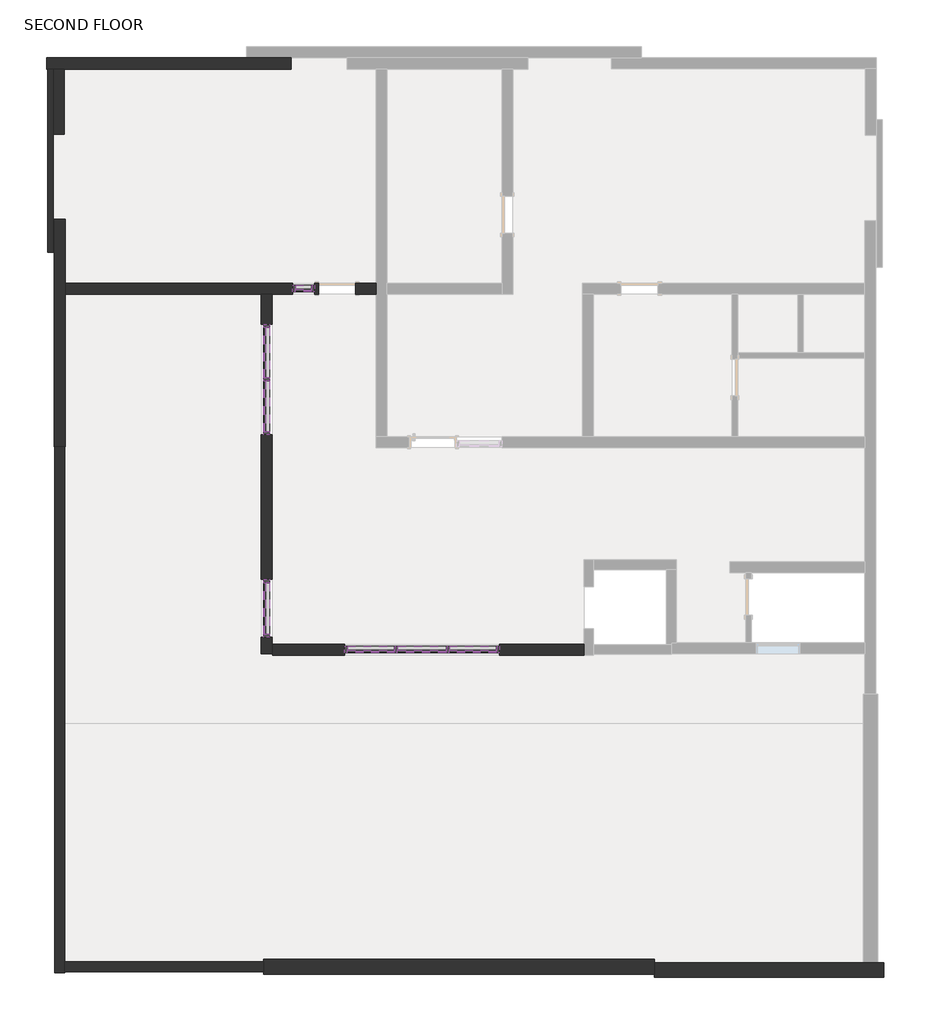
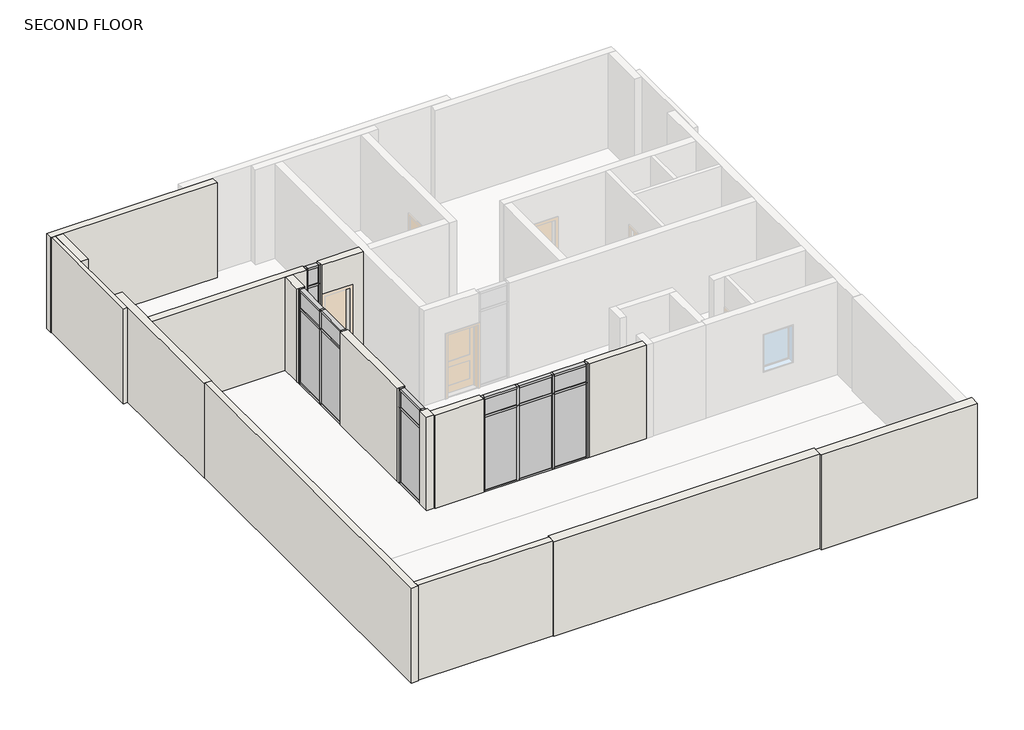
# One storey, part 1 of 2: 43 members, 14 plates, 11 walls.
"""IFC4 building model written with IfcOpenShell, lengths in millimetres."""

from ifc_helpers import new_model, si_unit, frame, origin, place, context, project, spatial, polyline, outline, extrude, faceted_brep, transform, mapped, element, save
from components import member_f0fea5a5, member_ee409385, member_c4de40ee, member_a715cb85, member_f03bb510, member_b0389538, member_0998ace5, member_b9dc02b9, member_6e77e263, member_47bfaf8a, member_78934672, member_697f972d, member_ff9f2d30, member_0c1408be, system_panel_glazed_daed1646, system_panel_glazed_43d75c16, system_panel_glazed_ee97838a, system_panel_glazed_b5d2153e, system_panel_glazed_ff9ba4bf, system_panel_glazed_ef7cd4ce, system_panel_glazed_cc935e45, system_panel_glazed_d41754d3, system_panel_glazed_720fdf88, system_panel_glazed_bfb04d77

model = new_model("IFC4")

# Units and contexts
model_context = context("Model", 3, world=origin())
ifc_project = project(units=[si_unit("LENGTHUNIT", "METRE", prefix="MILLI")], contexts=[model_context])

# Site, building, storey
site = spatial("IfcSite", under=ifc_project)
building = spatial("IfcBuilding", under=site)
storey = spatial("IfcBuildingStorey", under=building, Name="SECOND FLOOR", Elevation=6096.0)

# Members
placement = place(None, origin())
member_shape = member_f0fea5a5(model_context)
element("IfcMember", 1, ObjectType="Rectangular Mullion : 2.5\" x 5\" rectangular", at=placement, inside=storey, context=model_context, shape_type="MappedRepresentation", body=[
    mapped(member_shape, transform((2565.5464181, 4336.5216143, 6096.0), x_axis=(-1.0, 0.0, 0.0), y_axis=(0.0, 1.0, 0.0), z_axis=(0.0, 0.0, -1.0))),
])
element("IfcMember", 2, ObjectType="Rectangular Mullion : 2.5\" x 5\" rectangular", at=placement, inside=storey, context=model_context, shape_type="MappedRepresentation", body=[
    mapped(member_shape, transform((1498.7464183, 4336.5216143, 6096.0), x_axis=(-1.0, 0.0, 0.0), y_axis=(0.0, 1.0, 0.0), z_axis=(0.0, 0.0, -1.0))),
])
element("IfcMember", 3, ObjectType="Rectangular Mullion : 2.5\" x 5\" rectangular", at=placement, inside=storey, context=model_context, shape_type="MappedRepresentation", body=[
    mapped(member_shape, transform((-1181.6535114, 9915.8356247, 6096.0), x_axis=(0.0, 1.0, 0.0), y_axis=(1.0, 0.0, 0.0), z_axis=(0.0, 0.0, -1.0))),
])
member_2_shape = member_ee409385(model_context)
element("IfcMember", 4, ObjectType="Rectangular Mullion : 2.5\" x 5\" rectangular", at=placement, inside=storey, context=model_context, shape_type="MappedRepresentation", body=[
    mapped(member_2_shape, transform((431.9464182, 4336.5216143, 6096.0), x_axis=(-1.0, 0.0, 0.0), y_axis=(0.0, 1.0, 0.0), z_axis=(0.0, 0.0, -1.0))),
])
element("IfcMember", 5, ObjectType="Rectangular Mullion : 2.5\" x 5\" rectangular", at=placement, inside=storey, context=model_context, shape_type="MappedRepresentation", body=[
    mapped(member_2_shape, transform((-1181.6535114, 5784.3216143, 6096.0), x_axis=(0.0, 1.0, 0.0), y_axis=(1.0, 0.0, 0.0), z_axis=(0.0, 0.0, -1.0))),
])
element("IfcMember", 6, ObjectType="Rectangular Mullion : 2.5\" x 5\" rectangular", at=placement, inside=storey, context=model_context, shape_type="MappedRepresentation", body=[
    mapped(member_2_shape, transform((-1181.6535114, 11058.8356247, 6096.0), x_axis=(0.0, 1.0, 0.0), y_axis=(1.0, 0.0, 0.0), z_axis=(0.0, 0.0, -1.0))),
])
element("IfcMember", 7, ObjectType="Rectangular Mullion : 2.5\" x 5\" rectangular", at=placement, inside=storey, context=model_context, shape_type="MappedRepresentation", body=[
    mapped(member_2_shape, transform((-648.2535114, 11793.69348, 6096.0), x_axis=(-1.0, 0.0, 0.0), y_axis=(0.0, 1.0, 0.0), z_axis=(0.0, 0.0, -1.0))),
])
element("IfcMember", 8, ObjectType="Rectangular Mullion : 2.5\" x 5\" rectangular", at=placement, inside=storey, context=model_context, shape_type="MappedRepresentation", body=[
    mapped(member_2_shape, transform((3632.3464182, 4336.5216143, 8534.4), x_axis=(1.0, 0.0, 0.0), y_axis=(0.0, 1.0, 0.0), z_axis=(0.0, 0.0, 1.0))),
])
element("IfcMember", 9, ObjectType="Rectangular Mullion : 2.5\" x 5\" rectangular", at=placement, inside=storey, context=model_context, shape_type="MappedRepresentation", body=[
    mapped(member_2_shape, transform((-1181.6535114, 4590.5216143, 8534.4), x_axis=(0.0, -1.0, 0.0), y_axis=(1.0, 0.0, 0.0), z_axis=(0.0, 0.0, 1.0))),
])
element("IfcMember", 10, ObjectType="Rectangular Mullion : 2.5\" x 5\" rectangular", at=placement, inside=storey, context=model_context, shape_type="MappedRepresentation", body=[
    mapped(member_2_shape, transform((-1181.6535114, 8772.8356247, 8534.4), x_axis=(0.0, -1.0, 0.0), y_axis=(1.0, 0.0, 0.0), z_axis=(0.0, 0.0, 1.0))),
])
element("IfcMember", 11, ObjectType="Rectangular Mullion : 2.5\" x 5\" rectangular", at=placement, inside=storey, context=model_context, shape_type="MappedRepresentation", body=[
    mapped(member_2_shape, transform((-191.0535114, 11793.69348, 8534.4), x_axis=(1.0, 0.0, 0.0), y_axis=(0.0, 1.0, 0.0), z_axis=(0.0, 0.0, 1.0))),
])
member_3_shape = member_c4de40ee(model_context)
element("IfcMember", 12, ObjectType="Rectangular Mullion : 2.5\" x 5\" rectangular", at=placement, inside=storey, context=model_context, shape_type="MappedRepresentation", body=[
    mapped(member_3_shape, transform((-1181.6535114, 5720.8216143, 9144.0), x_axis=(0.0, 0.0, 1.0), y_axis=(1.0, 0.0, 0.0), z_axis=(0.0, 1.0, 0.0))),
])
element("IfcMember", 13, ObjectType="Rectangular Mullion : 2.5\" x 5\" rectangular", at=placement, inside=storey, context=model_context, shape_type="MappedRepresentation", body=[
    mapped(member_3_shape, transform((-1181.6535114, 4654.0216143, 6096.0), x_axis=(0.0, 0.0, -1.0), y_axis=(1.0, 0.0, 0.0), z_axis=(0.0, -1.0, 0.0))),
])
member_4_shape = member_a715cb85(model_context)
element("IfcMember", 14, ObjectType="Rectangular Mullion : 2.5\" x 5\" rectangular", at=placement, inside=storey, context=model_context, shape_type="MappedRepresentation", body=[
    mapped(member_4_shape, transform((-1181.6535114, 5720.8216143, 8534.4), x_axis=(0.0, 0.0, 1.0), y_axis=(1.0, 0.0, 0.0), z_axis=(0.0, 1.0, 0.0))),
])
member_5_shape = member_f03bb510(model_context)
element("IfcMember", 15, ObjectType="Rectangular Mullion : 2.5\" x 5\" rectangular", at=placement, inside=storey, context=model_context, shape_type="MappedRepresentation", body=[
    mapped(member_5_shape, transform((495.4464182, 4336.5216143, 9144.0), x_axis=(0.0, 0.0, 1.0), y_axis=(0.0, 1.0, 0.0), z_axis=(-1.0, 0.0, 0.0))),
])
element("IfcMember", 16, ObjectType="Rectangular Mullion : 2.5\" x 5\" rectangular", at=placement, inside=storey, context=model_context, shape_type="MappedRepresentation", body=[
    mapped(member_5_shape, transform((2597.2964181, 4336.5216143, 9144.0), x_axis=(0.0, 0.0, 1.0), y_axis=(0.0, 1.0, 0.0), z_axis=(-1.0, 0.0, 0.0))),
])
member_6_shape = member_b0389538(model_context)
element("IfcMember", 17, ObjectType="Rectangular Mullion : 2.5\" x 5\" rectangular", at=placement, inside=storey, context=model_context, shape_type="MappedRepresentation", body=[
    mapped(member_6_shape, transform((1530.4964183, 4336.5216143, 9144.0), x_axis=(0.0, 0.0, 1.0), y_axis=(0.0, 1.0, 0.0), z_axis=(-1.0, 0.0, 0.0))),
])
element("IfcMember", 18, ObjectType="Rectangular Mullion : 2.5\" x 5\" rectangular", at=placement, inside=storey, context=model_context, shape_type="MappedRepresentation", body=[
    mapped(member_5_shape, transform((3568.8464182, 4336.5216143, 6096.0), x_axis=(0.0, 0.0, -1.0), y_axis=(0.0, 1.0, 0.0), z_axis=(1.0, 0.0, 0.0))),
])
element("IfcMember", 19, ObjectType="Rectangular Mullion : 2.5\" x 5\" rectangular", at=placement, inside=storey, context=model_context, shape_type="MappedRepresentation", body=[
    mapped(member_5_shape, transform((1466.9964183, 4336.5216143, 6096.0), x_axis=(0.0, 0.0, -1.0), y_axis=(0.0, 1.0, 0.0), z_axis=(1.0, 0.0, 0.0))),
])
element("IfcMember", 20, ObjectType="Rectangular Mullion : 2.5\" x 5\" rectangular", at=placement, inside=storey, context=model_context, shape_type="MappedRepresentation", body=[
    mapped(member_6_shape, transform((2533.7964181, 4336.5216143, 6096.0), x_axis=(0.0, 0.0, -1.0), y_axis=(0.0, 1.0, 0.0), z_axis=(1.0, 0.0, 0.0))),
])
member_7_shape = member_0998ace5(model_context)
element("IfcMember", 21, ObjectType="Rectangular Mullion : 2.5\" x 5\" rectangular", at=placement, inside=storey, context=model_context, shape_type="MappedRepresentation", body=[
    mapped(member_7_shape, transform((2597.2964181, 4336.5216143, 8534.4), x_axis=(0.0, 0.0, 1.0), y_axis=(0.0, 1.0, 0.0), z_axis=(-1.0, 0.0, 0.0))),
])
element("IfcMember", 22, ObjectType="Rectangular Mullion : 2.5\" x 5\" rectangular", at=placement, inside=storey, context=model_context, shape_type="MappedRepresentation", body=[
    mapped(member_7_shape, transform((495.4464182, 4336.5216143, 8534.4), x_axis=(0.0, 0.0, 1.0), y_axis=(0.0, 1.0, 0.0), z_axis=(-1.0, 0.0, 0.0))),
])
member_8_shape = member_b9dc02b9(model_context)
element("IfcMember", 23, ObjectType="Rectangular Mullion : 2.5\" x 5\" rectangular", at=placement, inside=storey, context=model_context, shape_type="MappedRepresentation", body=[
    mapped(member_8_shape, transform((1530.4964183, 4336.5216143, 8534.4), x_axis=(0.0, 0.0, 1.0), y_axis=(0.0, 1.0, 0.0), z_axis=(-1.0, 0.0, 0.0))),
])
member_9_shape = member_6e77e263(model_context)
element("IfcMember", 24, ObjectType="Rectangular Mullion : 2.5\" x 5\" rectangular", at=placement, inside=storey, context=model_context, shape_type="MappedRepresentation", body=[
    mapped(member_9_shape, transform((2565.5464181, 4336.5216143, 8534.4), x_axis=(-1.0, 0.0, 0.0), y_axis=(0.0, 1.0, 0.0), z_axis=(0.0, 0.0, -1.0))),
])
element("IfcMember", 25, ObjectType="Rectangular Mullion : 2.5\" x 5\" rectangular", at=placement, inside=storey, context=model_context, shape_type="MappedRepresentation", body=[
    mapped(member_9_shape, transform((1498.7464183, 4336.5216143, 8534.4), x_axis=(-1.0, 0.0, 0.0), y_axis=(0.0, 1.0, 0.0), z_axis=(0.0, 0.0, -1.0))),
])
element("IfcMember", 26, ObjectType="Rectangular Mullion : 2.5\" x 5\" rectangular", at=placement, inside=storey, context=model_context, shape_type="MappedRepresentation", body=[
    mapped(member_9_shape, transform((-1181.6535114, 9915.8356247, 8534.4), x_axis=(0.0, 1.0, 0.0), y_axis=(1.0, 0.0, 0.0), z_axis=(0.0, 0.0, -1.0))),
])
member_10_shape = member_47bfaf8a(model_context)
element("IfcMember", 27, ObjectType="Rectangular Mullion : 2.5\" x 5\" rectangular", at=placement, inside=storey, context=model_context, shape_type="MappedRepresentation", body=[
    mapped(member_10_shape, transform((431.9464182, 4336.5216143, 8534.4), x_axis=(-1.0, 0.0, 0.0), y_axis=(0.0, 1.0, 0.0), z_axis=(0.0, 0.0, -1.0))),
])
element("IfcMember", 28, ObjectType="Rectangular Mullion : 2.5\" x 5\" rectangular", at=placement, inside=storey, context=model_context, shape_type="MappedRepresentation", body=[
    mapped(member_10_shape, transform((-1181.6535114, 5784.3216143, 8534.4), x_axis=(0.0, 1.0, 0.0), y_axis=(1.0, 0.0, 0.0), z_axis=(0.0, 0.0, -1.0))),
])
element("IfcMember", 29, ObjectType="Rectangular Mullion : 2.5\" x 5\" rectangular", at=placement, inside=storey, context=model_context, shape_type="MappedRepresentation", body=[
    mapped(member_10_shape, transform((-1181.6535114, 11058.8356247, 8534.4), x_axis=(0.0, 1.0, 0.0), y_axis=(1.0, 0.0, 0.0), z_axis=(0.0, 0.0, -1.0))),
])
element("IfcMember", 30, ObjectType="Rectangular Mullion : 2.5\" x 5\" rectangular", at=placement, inside=storey, context=model_context, shape_type="MappedRepresentation", body=[
    mapped(member_10_shape, transform((-648.2535114, 11793.69348, 8534.4), x_axis=(-1.0, 0.0, 0.0), y_axis=(0.0, 1.0, 0.0), z_axis=(0.0, 0.0, -1.0))),
])
element("IfcMember", 31, ObjectType="Rectangular Mullion : 2.5\" x 5\" rectangular", at=placement, inside=storey, context=model_context, shape_type="MappedRepresentation", body=[
    mapped(member_10_shape, transform((3632.3464182, 4336.5216143, 9144.0), x_axis=(1.0, 0.0, 0.0), y_axis=(0.0, 1.0, 0.0), z_axis=(0.0, 0.0, 1.0))),
])
element("IfcMember", 32, ObjectType="Rectangular Mullion : 2.5\" x 5\" rectangular", at=placement, inside=storey, context=model_context, shape_type="MappedRepresentation", body=[
    mapped(member_10_shape, transform((-1181.6535114, 4590.5216143, 9144.0), x_axis=(0.0, -1.0, 0.0), y_axis=(1.0, 0.0, 0.0), z_axis=(0.0, 0.0, 1.0))),
])
element("IfcMember", 33, ObjectType="Rectangular Mullion : 2.5\" x 5\" rectangular", at=placement, inside=storey, context=model_context, shape_type="MappedRepresentation", body=[
    mapped(member_10_shape, transform((-1181.6535114, 8772.8356247, 9144.0), x_axis=(0.0, -1.0, 0.0), y_axis=(1.0, 0.0, 0.0), z_axis=(0.0, 0.0, 1.0))),
])
element("IfcMember", 34, ObjectType="Rectangular Mullion : 2.5\" x 5\" rectangular", at=placement, inside=storey, context=model_context, shape_type="MappedRepresentation", body=[
    mapped(member_10_shape, transform((-191.0535114, 11793.69348, 9144.0), x_axis=(1.0, 0.0, 0.0), y_axis=(0.0, 1.0, 0.0), z_axis=(0.0, 0.0, 1.0))),
])
member_11_shape = member_78934672(model_context)
element("IfcMember", 35, ObjectType="Rectangular Mullion : 2.5\" x 5\" rectangular", at=placement, inside=storey, context=model_context, shape_type="MappedRepresentation", body=[
    mapped(member_11_shape, transform((-1181.6535114, 10995.3356247, 9144.0), x_axis=(0.0, 0.0, 1.0), y_axis=(1.0, 0.0, 0.0), z_axis=(0.0, 1.0, 0.0))),
])
element("IfcMember", 36, ObjectType="Rectangular Mullion : 2.5\" x 5\" rectangular", at=placement, inside=storey, context=model_context, shape_type="MappedRepresentation", body=[
    mapped(member_11_shape, transform((-1181.6535114, 9884.0856247, 9144.0), x_axis=(0.0, 0.0, 1.0), y_axis=(1.0, 0.0, 0.0), z_axis=(0.0, 1.0, 0.0))),
])
element("IfcMember", 37, ObjectType="Rectangular Mullion : 2.5\" x 5\" rectangular", at=placement, inside=storey, context=model_context, shape_type="MappedRepresentation", body=[
    mapped(member_11_shape, transform((-1181.6535114, 8836.3356247, 6096.0), x_axis=(0.0, 0.0, -1.0), y_axis=(1.0, 0.0, 0.0), z_axis=(0.0, -1.0, 0.0))),
])
element("IfcMember", 38, ObjectType="Rectangular Mullion : 2.5\" x 5\" rectangular", at=placement, inside=storey, context=model_context, shape_type="MappedRepresentation", body=[
    mapped(member_11_shape, transform((-1181.6535114, 9947.5856247, 6096.0), x_axis=(0.0, 0.0, -1.0), y_axis=(1.0, 0.0, 0.0), z_axis=(0.0, -1.0, 0.0))),
])
member_12_shape = member_697f972d(model_context)
element("IfcMember", 39, ObjectType="Rectangular Mullion : 2.5\" x 5\" rectangular", at=placement, inside=storey, context=model_context, shape_type="MappedRepresentation", body=[
    mapped(member_12_shape, transform((-1181.6535114, 9884.0856247, 8534.4), x_axis=(0.0, 0.0, 1.0), y_axis=(1.0, 0.0, 0.0), z_axis=(0.0, 1.0, 0.0))),
])
element("IfcMember", 40, ObjectType="Rectangular Mullion : 2.5\" x 5\" rectangular", at=placement, inside=storey, context=model_context, shape_type="MappedRepresentation", body=[
    mapped(member_12_shape, transform((-1181.6535114, 10995.3356247, 8534.4), x_axis=(0.0, 0.0, 1.0), y_axis=(1.0, 0.0, 0.0), z_axis=(0.0, 1.0, 0.0))),
])
member_13_shape = member_ff9f2d30(model_context)
element("IfcMember", 41, ObjectType="Rectangular Mullion : 2.5\" x 5\" rectangular", at=placement, inside=storey, context=model_context, shape_type="MappedRepresentation", body=[
    mapped(member_13_shape, transform((-584.7535114, 11793.69348, 9144.0), x_axis=(0.0, 0.0, 1.0), y_axis=(0.0, 1.0, 0.0), z_axis=(-1.0, 0.0, 0.0))),
])
element("IfcMember", 42, ObjectType="Rectangular Mullion : 2.5\" x 5\" rectangular", at=placement, inside=storey, context=model_context, shape_type="MappedRepresentation", body=[
    mapped(member_13_shape, transform((-254.5535114, 11793.69348, 6096.0), x_axis=(0.0, 0.0, -1.0), y_axis=(0.0, 1.0, 0.0), z_axis=(1.0, 0.0, 0.0))),
])
member_14_shape = member_0c1408be(model_context)
element("IfcMember", 43, ObjectType="Rectangular Mullion : 2.5\" x 5\" rectangular", at=placement, inside=storey, context=model_context, shape_type="MappedRepresentation", body=[
    mapped(member_14_shape, transform((-584.7535114, 11793.69348, 8534.4), x_axis=(0.0, 0.0, 1.0), y_axis=(0.0, 1.0, 0.0), z_axis=(-1.0, 0.0, 0.0))),
])

# Plates
system_panel_glazed_shape = system_panel_glazed_daed1646(model_context)
element("IfcPlate", 44, ObjectType="System Panel : Glazed", at=placement, inside=storey, context=model_context, shape_type="MappedRepresentation", body=[
    mapped(system_panel_glazed_shape, transform((-1181.6535114, 5187.4216143, 6159.5), x_axis=(0.0, 1.0, 0.0), y_axis=(-1.0, 0.0, 0.0), z_axis=(0.0, 0.0, 1.0))),
])
system_panel_glazed_2_shape = system_panel_glazed_43d75c16(model_context)
element("IfcPlate", 45, ObjectType="System Panel : Glazed", at=placement, inside=storey, context=model_context, shape_type="MappedRepresentation", body=[
    mapped(system_panel_glazed_2_shape, transform((3083.0714181, 4336.5216143, 6159.5), x_axis=(-1.0, 0.0, 0.0), y_axis=(0.0, -1.0, 0.0), z_axis=(0.0, 0.0, 1.0))),
])
element("IfcPlate", 46, ObjectType="System Panel : Glazed", at=placement, inside=storey, context=model_context, shape_type="MappedRepresentation", body=[
    mapped(system_panel_glazed_2_shape, transform((981.2214182, 4336.5216143, 6159.5), x_axis=(-1.0, 0.0, 0.0), y_axis=(0.0, -1.0, 0.0), z_axis=(0.0, 0.0, 1.0))),
])
system_panel_glazed_3_shape = system_panel_glazed_ee97838a(model_context)
element("IfcPlate", 47, ObjectType="System Panel : Glazed", at=placement, inside=storey, context=model_context, shape_type="MappedRepresentation", body=[
    mapped(system_panel_glazed_3_shape, transform((2032.1464182, 4336.5216143, 6159.5), x_axis=(-1.0, 0.0, 0.0), y_axis=(0.0, -1.0, 0.0), z_axis=(0.0, 0.0, 1.0))),
])
system_panel_glazed_4_shape = system_panel_glazed_b5d2153e(model_context)
element("IfcPlate", 48, ObjectType="System Panel : Glazed", at=placement, inside=storey, context=model_context, shape_type="MappedRepresentation", body=[
    mapped(system_panel_glazed_4_shape, transform((3083.0714181, 4336.5216143, 8566.15), x_axis=(-1.0, 0.0, 0.0), y_axis=(0.0, -1.0, 0.0), z_axis=(0.0, 0.0, 1.0))),
])
element("IfcPlate", 49, ObjectType="System Panel : Glazed", at=placement, inside=storey, context=model_context, shape_type="MappedRepresentation", body=[
    mapped(system_panel_glazed_4_shape, transform((981.2214182, 4336.5216143, 8566.15), x_axis=(-1.0, 0.0, 0.0), y_axis=(0.0, -1.0, 0.0), z_axis=(0.0, 0.0, 1.0))),
])
system_panel_glazed_5_shape = system_panel_glazed_ff9ba4bf(model_context)
element("IfcPlate", 50, ObjectType="System Panel : Glazed", at=placement, inside=storey, context=model_context, shape_type="MappedRepresentation", body=[
    mapped(system_panel_glazed_5_shape, transform((2032.1464182, 4336.5216143, 8566.15), x_axis=(-1.0, 0.0, 0.0), y_axis=(0.0, -1.0, 0.0), z_axis=(0.0, 0.0, 1.0))),
])
system_panel_glazed_6_shape = system_panel_glazed_ef7cd4ce(model_context)
element("IfcPlate", 51, ObjectType="System Panel : Glazed", at=placement, inside=storey, context=model_context, shape_type="MappedRepresentation", body=[
    mapped(system_panel_glazed_6_shape, transform((-1181.6535114, 5187.4216143, 8566.15), x_axis=(0.0, 1.0, 0.0), y_axis=(-1.0, 0.0, 0.0), z_axis=(0.0, 0.0, 1.0))),
])
system_panel_glazed_7_shape = system_panel_glazed_cc935e45(model_context)
element("IfcPlate", 52, ObjectType="System Panel : Glazed", at=placement, inside=storey, context=model_context, shape_type="MappedRepresentation", body=[
    mapped(system_panel_glazed_7_shape, transform((-1181.6535114, 9360.2106247, 6159.5), x_axis=(0.0, 1.0, 0.0), y_axis=(-1.0, 0.0, 0.0), z_axis=(0.0, 0.0, 1.0))),
])
element("IfcPlate", 53, ObjectType="System Panel : Glazed", at=placement, inside=storey, context=model_context, shape_type="MappedRepresentation", body=[
    mapped(system_panel_glazed_7_shape, transform((-1181.6535114, 10471.4606247, 6159.5), x_axis=(0.0, 1.0, 0.0), y_axis=(-1.0, 0.0, 0.0), z_axis=(0.0, 0.0, 1.0))),
])
system_panel_glazed_8_shape = system_panel_glazed_d41754d3(model_context)
element("IfcPlate", 54, ObjectType="System Panel : Glazed", at=placement, inside=storey, context=model_context, shape_type="MappedRepresentation", body=[
    mapped(system_panel_glazed_8_shape, transform((-1181.6535114, 9360.2106247, 8566.15), x_axis=(0.0, 1.0, 0.0), y_axis=(-1.0, 0.0, 0.0), z_axis=(0.0, 0.0, 1.0))),
])
element("IfcPlate", 55, ObjectType="System Panel : Glazed", at=placement, inside=storey, context=model_context, shape_type="MappedRepresentation", body=[
    mapped(system_panel_glazed_8_shape, transform((-1181.6535114, 10471.4606247, 8566.15), x_axis=(0.0, 1.0, 0.0), y_axis=(-1.0, 0.0, 0.0), z_axis=(0.0, 0.0, 1.0))),
])
system_panel_glazed_9_shape = system_panel_glazed_720fdf88(model_context)
element("IfcPlate", 56, ObjectType="System Panel : Glazed", at=placement, inside=storey, context=model_context, shape_type="MappedRepresentation", body=[
    mapped(system_panel_glazed_9_shape, transform((-419.6535114, 11793.69348, 6159.5), x_axis=(-1.0, 0.0, 0.0), y_axis=(0.0, -1.0, 0.0), z_axis=(0.0, 0.0, 1.0))),
])
system_panel_glazed_10_shape = system_panel_glazed_bfb04d77(model_context)
element("IfcPlate", 57, ObjectType="System Panel : Glazed", at=placement, inside=storey, context=model_context, shape_type="MappedRepresentation", body=[
    mapped(system_panel_glazed_10_shape, transform((-419.6535114, 11793.69348, 8566.15), x_axis=(-1.0, 0.0, 0.0), y_axis=(0.0, -1.0, 0.0), z_axis=(0.0, 0.0, 1.0))),
])

# Walls
element("IfcWall", 58, ObjectType="INNER WALL 4.5\"", at=placement, inside=storey, context=model_context, shape_type="SweptSolid", body=[
    extrude(outline(polyline([(-5594.7327494, 16327.59348), (-5594.7327494, 12547.6213266), (-5709.0327494, 12547.6213266), (-5709.0327494, 16327.59348), (-5594.7327494, 16327.59348)])), frame((0.0, 0.0, 6096.0), z_axis=(0.0, 0.0, 1.0), x_axis=(1.0, 0.0, 0.0)), (0.0, 0.0, 1.0), 3048.0),
])
element("IfcWall", 59, ObjectType="OUTER WALL THICKNESS 8\"", at=placement, inside=storey, context=model_context, shape_type="Brep", body=[
    faceted_brep([(-5560.894009, 8528.9097639, 6096.0), (-5560.894009, -2342.2902361, 6096.0), (-5560.894009, -2342.2902361, 9144.0), (-5560.894009, 8528.9097639, 9144.0), (-5357.694009, 8528.9097639, 6096.0), (-5357.694009, 8528.9097639, 9144.0), (-5357.694009, -2113.6902361, 9144.0), (-5357.694009, -2316.8902361, 9144.0), (-5357.694009, -2342.2902361, 9144.0), (-5357.694009, -2342.2902361, 6096.0), (-5357.694009, -2316.8902361, 6096.0), (-5357.694009, -2113.6902361, 6096.0)], [[[0, 1, 2, 3]], [[4, 5, 6, 7, 8, 9, 10, 11]], [[1, 0, 4, 11, 10, 9]], [[2, 1, 9, 8]], [[3, 2, 8, 7, 6, 5]], [[0, 3, 5, 4]]]),
])
element("IfcWall", 60, ObjectType="OUTER WALL THICKNESS 8\"", at=placement, inside=storey, context=model_context, shape_type="SweptSolid", body=[
    extrude(outline(polyline([(-1242.894009, -2316.8902361), (-5357.694009, -2316.8902361), (-5357.694009, -2113.6902361), (-1242.894009, -2113.6902361), (-1242.894009, -2316.8902361)])), frame((0.0, 0.0, 6096.0), z_axis=(0.0, 0.0, 1.0), x_axis=(1.0, 0.0, 0.0)), (0.0, 0.0, 1.0), 3048.0),
])
element("IfcWall", 61, ObjectType="OUTER WALL THICKNESS 9\"", at=placement, inside=storey, context=model_context, shape_type="Brep", body=[
    faceted_brep([(-674.5187543, 16556.19348, 6096.0), (-5729.1187543, 16556.19348, 6096.0), (-5729.1187543, 16556.19348, 9144.0), (-674.5187543, 16556.19348, 9144.0), (-674.5187543, 16327.59348, 6096.0), (-674.5187543, 16327.59348, 9144.0), (-5364.044009, 16327.59348, 9144.0), (-5592.644009, 16327.59348, 9144.0), (-5594.7327494, 16327.59348, 9144.0), (-5709.0327494, 16327.59348, 9144.0), (-5729.1187543, 16327.59348, 9144.0), (-5729.1187543, 16327.59348, 6096.0), (-5709.0327494, 16327.59348, 6096.0), (-5594.7327494, 16327.59348, 6096.0), (-5592.644009, 16327.59348, 6096.0), (-5364.044009, 16327.59348, 6096.0)], [[[0, 1, 2, 3]], [[4, 5, 6, 7, 8, 9, 10, 11, 12, 13, 14, 15]], [[1, 0, 4, 15, 14, 13, 12, 11]], [[2, 1, 11, 10]], [[3, 2, 10, 9, 8, 7, 6, 5]], [[0, 3, 5, 4]]]),
])
element("IfcWall", 62, ObjectType="OUTER WALL THICKNESS 9\"", at=placement, inside=storey, context=model_context, shape_type="SweptSolid", body=[
    extrude(outline(polyline([(-5592.644009, 14981.39348), (-5592.644009, 16327.59348), (-5364.044009, 16327.59348), (-5364.044009, 14981.39348), (-5592.644009, 14981.39348)])), frame((0.0, 0.0, 6096.0), z_axis=(0.0, 0.0, 1.0), x_axis=(1.0, 0.0, 0.0)), (0.0, 0.0, 1.0), 3048.0),
])
element("IfcWall", 63, ObjectType="OUTER WALL THICKNESS 9\"", at=placement, inside=storey, context=model_context, shape_type="Brep", body=[
    faceted_brep([(-5573.594009, 13227.9097639, 6096.0), (-5573.594009, 8528.9097639, 6096.0), (-5573.594009, 8528.9097639, 9144.0), (-5573.594009, 13227.9097639, 9144.0), (-5344.994009, 13227.9097639, 6096.0), (-5344.994009, 13227.9097639, 9144.0), (-5344.994009, 11907.99348, 9144.0), (-5344.994009, 11679.39348, 9144.0), (-5344.994009, 8528.9097639, 9144.0), (-5344.994009, 8528.9097639, 6096.0), (-5344.994009, 11679.39348, 6096.0), (-5344.994009, 11907.99348, 6096.0), (-5357.694009, 8528.9097639, 6096.0), (-5560.894009, 8528.9097639, 6096.0), (-5357.694009, 8528.9097639, 9144.0), (-5560.894009, 8528.9097639, 9144.0)], [[[0, 1, 2, 3]], [[4, 5, 6, 7, 8, 9, 10, 11]], [[1, 0, 4, 11, 10, 9, 12, 13]], [[2, 1, 13, 12, 9, 8, 14, 15]], [[3, 2, 15, 14, 8, 7, 6, 5]], [[0, 3, 5, 4]]]),
])
element("IfcWall", 64, ObjectType="OUTER WALL THICKNESS 9\"", at=placement, inside=storey, context=model_context, shape_type="Brep", body=[
    faceted_brep([(1076.9068953, 11679.39348, 6096.0), (1076.9068953, 11679.39348, 9144.0), (-191.0535114, 11679.39348, 9144.0), (-191.0535114, 11679.39348, 6096.0), (-104.1931047, 11679.39348, 6096.0), (-104.1931047, 11679.39348, 8128.0), (657.8068953, 11679.39348, 8128.0), (657.8068953, 11679.39348, 6096.0), (1076.9068953, 11907.99348, 9144.0), (1076.9068953, 11907.99348, 6096.0), (657.8068953, 11907.99348, 6096.0), (657.8068953, 11907.99348, 8128.0), (-104.1931047, 11907.99348, 8128.0), (-104.1931047, 11907.99348, 6096.0), (-191.0535114, 11907.99348, 6096.0), (-191.0535114, 11907.99348, 9144.0)], [[[0, 1, 2, 3, 4, 5, 6, 7]], [[8, 9, 10, 11, 12, 13, 14, 15]], [[9, 0, 7, 10]], [[13, 4, 3, 14]], [[1, 8, 15, 2]], [[1, 0, 9, 8]], [[11, 10, 7, 6]], [[12, 11, 6, 5]], [[13, 12, 5, 4]], [[3, 2, 15, 14]]]),
    faceted_brep([(-5344.994009, 11679.39348, 9144.0), (-5344.994009, 11679.39348, 6096.0), (-1295.9535114, 11679.39348, 6096.0), (-1067.3535114, 11679.39348, 6096.0), (-648.2535114, 11679.39348, 6096.0), (-648.2535114, 11679.39348, 9144.0), (-1067.3535114, 11679.39348, 9144.0), (-1295.9535114, 11679.39348, 9144.0), (-5344.994009, 11907.99348, 6096.0), (-5344.994009, 11907.99348, 9144.0), (-648.2535114, 11907.99348, 9144.0), (-648.2535114, 11907.99348, 6096.0)], [[[0, 1, 2, 3, 4, 5, 6, 7]], [[8, 9, 10, 11]], [[1, 8, 11, 4, 3, 2]], [[9, 0, 7, 6, 5, 10]], [[1, 0, 9, 8]], [[5, 4, 11, 10]]]),
])
element("IfcWall", 65, ObjectType="OUTER WALL THICKNESS 9\"", at=placement, inside=storey, context=model_context, shape_type="SweptSolid", body=[
    extrude(outline(polyline([(-1067.3535114, 4249.89348), (-1295.9535114, 4249.89348), (-1295.9535114, 4590.5216143), (-1067.3535114, 4590.5216143), (-1067.3535114, 4249.89348)])), frame((0.0, 0.0, 6096.0), z_axis=(0.0, 0.0, 1.0), x_axis=(1.0, 0.0, 0.0)), (0.0, 0.0, 1.0), 3048.0),
    extrude(outline(polyline([(-1295.9535114, 11679.39348), (-1067.3535114, 11679.39348), (-1067.3535114, 11058.8356247), (-1295.9535114, 11058.8356247), (-1295.9535114, 11679.39348)])), frame((0.0, 0.0, 6096.0), z_axis=(0.0, 0.0, 1.0), x_axis=(1.0, 0.0, 0.0)), (0.0, 0.0, 1.0), 3048.0),
    extrude(outline(polyline([(-1067.3535114, 5784.3216143), (-1295.9535114, 5784.3216143), (-1295.9535114, 8772.8356247), (-1067.3535114, 8772.8356247), (-1067.3535114, 5784.3216143)])), frame((0.0, 0.0, 6096.0), z_axis=(0.0, 0.0, 1.0), x_axis=(1.0, 0.0, 0.0)), (0.0, 0.0, 1.0), 3048.0),
])
element("IfcWall", 66, ObjectType="OUTER WALL THICKNESS 9\"", at=placement, inside=storey, context=model_context, shape_type="SweptSolid", body=[
    extrude(outline(polyline([(-1059.3262442, 4222.2216143), (-1059.3262442, 4450.8216143), (431.9464182, 4450.8216143), (431.9464182, 4222.2216143), (-1059.3262442, 4222.2216143)])), frame((0.0, 0.0, 6096.0), z_axis=(0.0, 0.0, 1.0), x_axis=(1.0, 0.0, 0.0)), (0.0, 0.0, 1.0), 3048.0),
    extrude(outline(polyline([(5375.3606323, 4450.8216143), (5375.3606323, 4222.2216143), (3632.3464182, 4222.2216143), (3632.3464182, 4450.8216143), (5375.3606323, 4450.8216143)])), frame((0.0, 0.0, 6096.0), z_axis=(0.0, 0.0, 1.0), x_axis=(1.0, 0.0, 0.0)), (0.0, 0.0, 1.0), 3048.0),
])
element("IfcWall", 67, ObjectType="WALL THICKNESS 1'", at=placement, inside=storey, context=model_context, shape_type="Brep", body=[
    faceted_brep([(-1242.894009, -2367.6902361, 6096.0), (6834.305991, -2367.6902361, 6096.0), (6834.305991, -2367.6902361, 9144.0), (-1242.894009, -2367.6902361, 9144.0), (-1242.894009, -2062.8902361, 6096.0), (-1242.894009, -2062.8902361, 9144.0), (6834.305991, -2062.8902361, 9144.0), (6834.305991, -2062.8902361, 6096.0), (-1242.894009, -2316.8902361, 6096.0), (-1242.894009, -2113.6902361, 6096.0), (6834.305991, -2132.117542, 6096.0), (6834.305991, -2132.117542, 9144.0), (-1242.894009, -2113.6902361, 9144.0), (-1242.894009, -2316.8902361, 9144.0)], [[[0, 1, 2, 3]], [[4, 5, 6, 7]], [[1, 0, 8, 9, 4, 7, 10]], [[2, 1, 10, 7, 6, 11]], [[3, 2, 11, 6, 5, 12, 13]], [[0, 3, 13, 12, 5, 4, 9, 8]]]),
])
element("IfcWall", 68, ObjectType="WALL THICKNESS 1'", at=placement, inside=storey, context=model_context, shape_type="Brep", body=[
    faceted_brep([(6834.305991, -2436.917542, 6096.0), (11579.9862453, -2436.917542, 6096.0), (11579.9862453, -2436.917542, 9144.0), (6834.305991, -2436.917542, 9144.0), (6834.305991, -2132.117542, 6096.0), (6834.305991, -2132.117542, 9144.0), (11147.3141504, -2132.117542, 9144.0), (11452.1141504, -2132.117542, 9144.0), (11579.9862453, -2132.117542, 9144.0), (11579.9862453, -2132.117542, 6096.0), (11452.1141504, -2132.117542, 6096.0), (11147.3141504, -2132.117542, 6096.0), (6834.305991, -2367.6902361, 6096.0), (6834.305991, -2367.6902361, 9144.0)], [[[0, 1, 2, 3]], [[4, 5, 6, 7, 8, 9, 10, 11]], [[1, 0, 12, 4, 11, 10, 9]], [[2, 1, 9, 8]], [[3, 2, 8, 7, 6, 5, 13]], [[0, 3, 13, 5, 4, 12]]]),
])

save(model, "model.ifc")

# Revit data of these elements
# Type "Rectangular Mullion : 2.5\" x 5\" rectangular"
#   built-in parameter 1007304 = 0.416667 (stored number, unit not read)
#   built-in parameter 1007301 = 0.104167 (stored number, unit not read)
#   built-in parameter 1007300 = 0.104167 (stored number, unit not read)
# Type "System Panel : Glazed"
#   Construction Type Id = "GSP4R"
#   Analytic Construction = "1/8 in Pilkington single glazing"
#   Visual Light Transmittance = 0.9
#   Solar Heat Gain Coefficient = 0.86
#   Heat Transfer Coefficient (U) = 1.18115 BTU/(h·ft²·°F)
#   Define Thermal Properties by = 1
# Type "INNER WALL 4.5\""
#   Assembly Code = "B2010"
#   Layers, outside or top first: 0' - 4 1/2" "BEIGE COLOUR" (function 1)
# Type "OUTER WALL THICKNESS 8\""
#   Assembly Code = "B2010"
#   Layers, outside or top first: 0' - 8" "BEIGE COLOUR" (function 1)
# Type "OUTER WALL THICKNESS 9\""
#   Assembly Code = "B2010"
#   Layers, outside or top first: 0' - 9" "BEIGE COLOUR" (function 1)
# Type "WALL THICKNESS 1'"
#   Assembly Code = "B2010"
#   Layers, outside or top first: 1' - 0" "BEIGE COLOUR" (function 1)
# Elements 1, 2, 3, 4, 5, 6, 7, 8, 9, 10, 11, 12, 13, 14, 15, 16, 17, 18, 19, 20, 21, 22, 23, 24, 25, 26, 27, 28, 29, 30, 31, 32, 33, 34, 35, 36, 37, 38, 39, 40, 41, 42, 43 (IfcMember, "Rectangular Mullion : 2.5\" x 5\" rectangular")
#   Phase Created = New Construction
#   Materials on its faces: "Aluminum"
# Elements 44, 45, 46, 47, 48, 49, 50, 51, 52, 53, 54, 55, 56, 57 (IfcPlate, "System Panel : Glazed")
#   Phase Created = New Construction
#   Materials on its faces: "Glass"
# Element 58 (IfcWall, "INNER WALL 4.5\"")
#   Top Offset = 0' - 0"
#   Base Offset = 0' - 0"
#   wall height = 10' - 0"
#   Phase Created = New Construction
#   Base Constraint = SECOND FLOOR
#   Top Constraint = TOP OF ROOFING
#   Materials on its faces: "BEIGE COLOUR"
# Elements 59, 60 (IfcWall, "OUTER WALL THICKNESS 8\"")
#   Top Offset = 0' - 0"
#   Base Offset = 0' - 0"
#   wall height = 10' - 0"
#   Phase Created = New Construction
#   Base Constraint = SECOND FLOOR
#   Top Constraint = TOP OF ROOFING
#   Materials on its faces: "BEIGE COLOUR"
# Elements 61, 62, 63, 64, 65, 66 (IfcWall, "OUTER WALL THICKNESS 9\"")
#   Top Offset = 0' - 0"
#   Base Offset = 0' - 0"
#   wall height = 10' - 0"
#   Phase Created = New Construction
#   Base Constraint = SECOND FLOOR
#   Top Constraint = TOP OF ROOFING
#   Materials on its faces: "BEIGE COLOUR"
# Elements 67, 68 (IfcWall, "WALL THICKNESS 1'")
#   Top Offset = 0' - 0"
#   Base Offset = 0' - 0"
#   wall height = 10' - 0"
#   Phase Created = New Construction
#   Base Constraint = SECOND FLOOR
#   Top Constraint = TOP OF ROOFING
#   Materials on its faces: "BEIGE COLOUR"
# Materials
#   "BEIGE COLOUR": class "Generic", colour RGB 120 120 120, transparency 0, Cost = 0
#   "Aluminum": class "Metal", colour RGB 247 247 247, transparency 0, Description = "Aluminum 6061", Cost = 0
#   "Glass": class "Glass", colour RGB 0 128 192, transparency 0.75, Description = "Soda Lime Glass", Cost = 0
